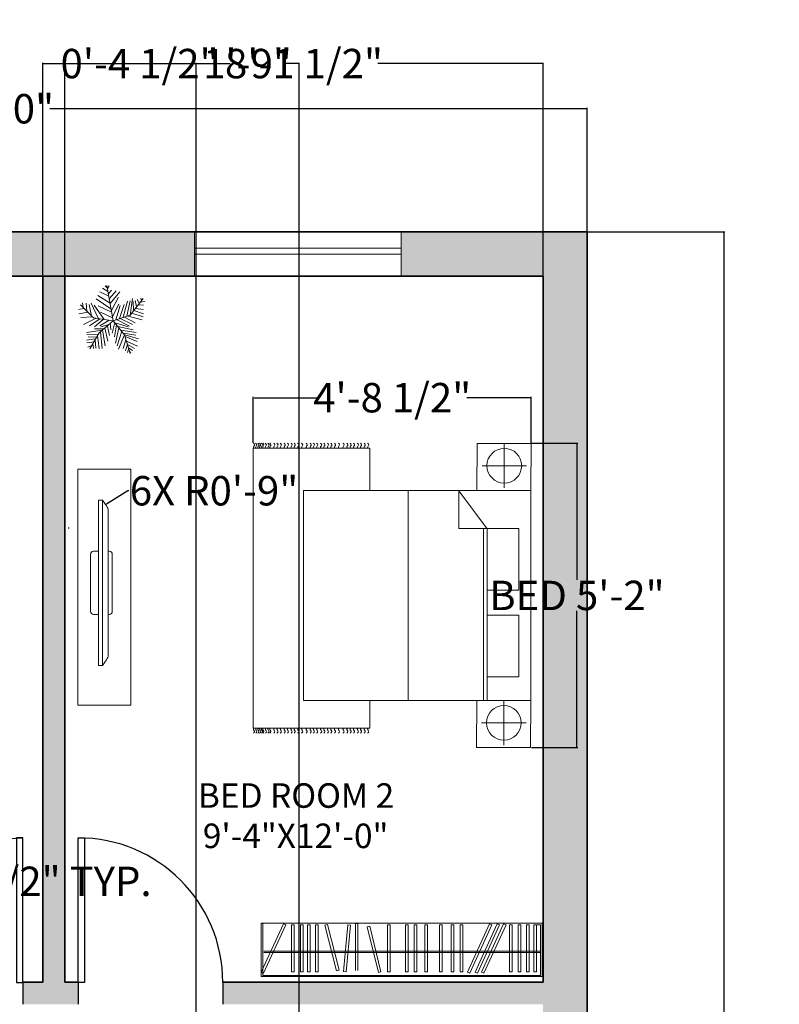
# Model space of a CAD drawing. Units: inches. Extents: x 143233372 to 143233714, y 112671713 to 112672292.
# Tile 7 of 7: x 143233541 to 143233695, y 112672092 to 112672292. Entities that reach past the tile are written whole.
import ezdxf

# ---------------------------------------------------------------- set-up
doc = ezdxf.new("R2010")
doc.units = ezdxf.units.IN
doc.header["$MEASUREMENT"] = 0
doc.layers.get('0').update_dxf_attribs({"color": 104})
for name, color, linetype, lineweight in [('A-ANNO-DIMS', 2, 'Continuous', 18), ('A-AREA-IDEN', 7, 'Continuous', 18), ('A-EQPM', 8, 'Continuous', 18), ('closet', 23, 'Continuous', 18), ('doors', 32, 'Continuous', 25), ('furniture', 23, 'Continuous', 18), ('L-PLNT', 92, 'Continuous', 13), ('walls', 7, 'Continuous', 35), ('windows', 4, 'Continuous', 18)]:
    doc.layers.add(name, color=color, linetype=linetype, lineweight=lineweight)
doc.layers.add('A-WALL-PATT', color=18, linetype='Continuous', lineweight=9, true_color=0x000000)
doc.styles.get("Standard").update_dxf_attribs({"font": 'arial.ttf'})
doc.dimstyles.get("Standard").update_dxf_attribs({"dimtxt": 6, "dimasz": 0.18, "dimexe": 0.18, "dimexo": 0.0625, "dimgap": 0.09, "dimtad": 0, "dimtih": 1, "dimtoh": 1, "dimzin": 0, "dimdsep": 46, "dimlunit": 3, "dimtxsty": 'Standard', "dimcen": 0.09, "dimadec": 0, "dimazin": 0, "dimtfac": 1, "dimtofl": 0, "dimtmove": 0, "dimatfit": 3, "dimfxl": 1, "dimtolj": 1, "dimtzin": 0, "dimarcsym": 0})

# ---------------------------------------------------------------- blocks, each defined once
blk = doc.blocks.new('PLASMA-LARGE')
at = {"layer": 'furniture'}
for p, q in [((-7.26, 0), (7.26, 0)), ((-21, -2.5), (21, -2.5)), ((-21, -2.5), (-21, -3.5)), ((-18.61, -1), (18.61, -1)), ((-8, -1), (-8, -0.74)), ((8, -1), (8, -0.74)), ((21, -2.5), (21, -3.5)), ((-21, -3.5), (21, -3.5)), ((-8, -3.5), (-8, -4.76)), ((8, -3.5), (8, -4.76)), ((-7.26, -5.5), (7.26, -5.5))]:
    blk.add_line(p, q, dxfattribs=at)
for centre, radius, start, end in [((-7.26, -0.74), 0.744, 90, 180), ((7.26, -0.74), 0.744, 0, 90), ((-13.97, -11.05), 11.07, 114.7602, 129.4175), ((13.97, -11.05), 11.07, 50.5825, 65.2398), ((-7.26, -4.76), 0.744, 180, 270), ((7.26, -4.76), 0.744, 270, 0)]:
    blk.add_arc(centre, radius, start, end, dxfattribs=at)
blk = doc.blocks.new('CARPET')
at = {"layer": 'furniture'}
for p, q in [((-51.53, -98.11), (-51.53, -55.12)), ((-51.53, -55.12), (-41.27, -55.12)), ((36, -55.12), (51.55, -55.12)), ((51.55, -55.12), (51.55, -98.11)), ((51.55, -98.11), (-51.53, -98.11))]:
    blk.add_line(p, q, dxfattribs=at)
for points, knots in [([(-53.37, -55.99), (-53.22, -55.8), (-52.9, -55.41), (-52.34, -55.8), (-51.89, -56.08), (-51.65, -55.91), (-51.53, -55.83)], [0, 0, 0, 0, 0.653278, 1.290138, 1.740457, 2.114451, 2.114451, 2.114451, 2.114451]), ([(-53.37, -57.26), (-53.22, -57.07), (-52.9, -56.67), (-52.34, -57.07), (-51.89, -57.35), (-51.65, -57.17), (-51.53, -57.1)], [0, 0, 0, 0, 0.653278, 1.290138, 1.740457, 2.114451, 2.114451, 2.114451, 2.114451]), ([(53.37, -55.99), (53.22, -55.8), (52.9, -55.41), (52.34, -55.8), (51.89, -56.08), (51.65, -55.91), (51.53, -55.83)], [0, 0, 0, 0, 0.653278, 1.290138, 1.740457, 2.114451, 2.114451, 2.114451, 2.114451]), ([(53.37, -57.26), (53.22, -57.07), (52.9, -56.67), (52.34, -57.07), (51.89, -57.35), (51.65, -57.17), (51.53, -57.1)], [0, 0, 0, 0, 0.653278, 1.290138, 1.740457, 2.114451, 2.114451, 2.114451, 2.114451]), ([(-53.37, -58.59), (-53.22, -58.4), (-52.9, -58.01), (-52.34, -58.4), (-51.89, -58.68), (-51.65, -58.5), (-51.53, -58.43)], [0, 0, 0, 0, 0.653278, 1.290138, 1.740457, 2.114451, 2.114451, 2.114451, 2.114451]), ([(-53.37, -59.78), (-53.22, -59.58), (-52.9, -59.19), (-52.34, -59.58), (-51.89, -59.86), (-51.65, -59.69), (-51.53, -59.61)], [0, 0, 0, 0, 0.653278, 1.290138, 1.740457, 2.114451, 2.114451, 2.114451, 2.114451]), ([(-53.37, -61.22), (-53.22, -61.02), (-52.9, -60.63), (-52.34, -61.02), (-51.89, -61.3), (-51.65, -61.13), (-51.53, -61.05)], [0, 0, 0, 0, 0.653278, 1.290138, 1.740457, 2.114451, 2.114451, 2.114451, 2.114451]), ([(53.37, -58.59), (53.22, -58.4), (52.9, -58.01), (52.34, -58.4), (51.89, -58.68), (51.65, -58.5), (51.53, -58.43)], [0, 0, 0, 0, 0.653278, 1.290138, 1.740457, 2.114451, 2.114451, 2.114451, 2.114451]), ([(53.37, -59.78), (53.22, -59.58), (52.9, -59.19), (52.34, -59.58), (51.89, -59.86), (51.65, -59.69), (51.53, -59.61)], [0, 0, 0, 0, 0.653278, 1.290138, 1.740457, 2.114451, 2.114451, 2.114451, 2.114451]), ([(53.37, -61.22), (53.22, -61.02), (52.9, -60.63), (52.34, -61.02), (51.89, -61.3), (51.65, -61.13), (51.53, -61.05)], [0, 0, 0, 0, 0.653278, 1.290138, 1.740457, 2.114451, 2.114451, 2.114451, 2.114451]), ([(-53.37, -62.44), (-53.22, -62.25), (-52.9, -61.86), (-52.34, -62.25), (-51.89, -62.53), (-51.65, -62.36), (-51.53, -62.28)], [0, 0, 0, 0, 0.653278, 1.290138, 1.740457, 2.114451, 2.114451, 2.114451, 2.114451]), ([(-53.37, -63.63), (-53.22, -63.43), (-52.9, -63.04), (-52.34, -63.43), (-51.89, -63.72), (-51.65, -63.54), (-51.53, -63.46)], [0, 0, 0, 0, 0.653278, 1.290138, 1.740457, 2.114451, 2.114451, 2.114451, 2.114451]), ([(-53.37, -65.07), (-53.22, -64.87), (-52.9, -64.48), (-52.34, -64.87), (-51.89, -65.15), (-51.65, -64.98), (-51.53, -64.9)], [0, 0, 0, 0, 0.653278, 1.290138, 1.740457, 2.114451, 2.114451, 2.114451, 2.114451]), ([(53.37, -62.44), (53.22, -62.25), (52.9, -61.86), (52.34, -62.25), (51.89, -62.53), (51.65, -62.36), (51.53, -62.28)], [0, 0, 0, 0, 0.653278, 1.290138, 1.740457, 2.114451, 2.114451, 2.114451, 2.114451]), ([(53.37, -63.63), (53.22, -63.43), (52.9, -63.04), (52.34, -63.43), (51.89, -63.72), (51.65, -63.54), (51.53, -63.46)], [0, 0, 0, 0, 0.653278, 1.290138, 1.740457, 2.114451, 2.114451, 2.114451, 2.114451]), ([(53.37, -65.07), (53.22, -64.87), (52.9, -64.48), (52.34, -64.87), (51.89, -65.15), (51.65, -64.98), (51.53, -64.9)], [0, 0, 0, 0, 0.653278, 1.290138, 1.740457, 2.114451, 2.114451, 2.114451, 2.114451]), ([(-53.37, -66.76), (-53.22, -66.56), (-52.9, -66.17), (-52.34, -66.56), (-51.89, -66.84), (-51.65, -66.67), (-51.53, -66.59)], [0, 0, 0, 0, 0.653278, 1.290138, 1.740457, 2.114451, 2.114451, 2.114451, 2.114451]), ([(-53.37, -68.2), (-53.22, -68), (-52.9, -67.61), (-52.34, -68), (-51.89, -68.28), (-51.65, -68.11), (-51.53, -68.03)], [0, 0, 0, 0, 0.653278, 1.290138, 1.740457, 2.114451, 2.114451, 2.114451, 2.114451]), ([(53.37, -66.76), (53.22, -66.56), (52.9, -66.17), (52.34, -66.56), (51.89, -66.84), (51.65, -66.67), (51.53, -66.59)], [0, 0, 0, 0, 0.653278, 1.290138, 1.740457, 2.114451, 2.114451, 2.114451, 2.114451]), ([(53.37, -68.2), (53.22, -68), (52.9, -67.61), (52.34, -68), (51.89, -68.28), (51.65, -68.11), (51.53, -68.03)], [0, 0, 0, 0, 0.653278, 1.290138, 1.740457, 2.114451, 2.114451, 2.114451, 2.114451]), ([(-53.37, -69.53), (-53.22, -69.33), (-52.9, -68.94), (-52.34, -69.33), (-51.89, -69.61), (-51.65, -69.44), (-51.53, -69.36)], [0, 0, 0, 0, 0.653278, 1.290138, 1.740457, 2.114451, 2.114451, 2.114451, 2.114451]), ([(-53.37, -70.79), (-53.22, -70.6), (-52.9, -70.21), (-52.34, -70.6), (-51.89, -70.88), (-51.65, -70.7), (-51.53, -70.63)], [0, 0, 0, 0, 0.653278, 1.290138, 1.740457, 2.114451, 2.114451, 2.114451, 2.114451]), ([(-53.37, -72.12), (-53.22, -71.93), (-52.9, -71.54), (-52.34, -71.93), (-51.89, -72.21), (-51.65, -72.04), (-51.53, -71.96)], [0, 0, 0, 0, 0.653278, 1.290138, 1.740457, 2.114451, 2.114451, 2.114451, 2.114451]), ([(53.37, -69.53), (53.22, -69.33), (52.9, -68.94), (52.34, -69.33), (51.89, -69.61), (51.65, -69.44), (51.53, -69.36)], [0, 0, 0, 0, 0.653278, 1.290138, 1.740457, 2.114451, 2.114451, 2.114451, 2.114451]), ([(53.37, -70.79), (53.22, -70.6), (52.9, -70.21), (52.34, -70.6), (51.89, -70.88), (51.65, -70.7), (51.53, -70.63)], [0, 0, 0, 0, 0.653278, 1.290138, 1.740457, 2.114451, 2.114451, 2.114451, 2.114451]), ([(53.37, -72.12), (53.22, -71.93), (52.9, -71.54), (52.34, -71.93), (51.89, -72.21), (51.65, -72.04), (51.53, -71.96)], [0, 0, 0, 0, 0.653278, 1.290138, 1.740457, 2.114451, 2.114451, 2.114451, 2.114451]), ([(-53.37, -73.31), (-53.22, -73.11), (-52.9, -72.72), (-52.34, -73.11), (-51.89, -73.4), (-51.65, -73.22), (-51.53, -73.14)], [0, 0, 0, 0, 0.653278, 1.290138, 1.740457, 2.114451, 2.114451, 2.114451, 2.114451]), ([(-53.37, -74.75), (-53.22, -74.55), (-52.9, -74.16), (-52.34, -74.55), (-51.89, -74.83), (-51.65, -74.66), (-51.53, -74.58)], [0, 0, 0, 0, 0.653278, 1.290138, 1.740457, 2.114451, 2.114451, 2.114451, 2.114451]), ([(-53.37, -75.98), (-53.22, -75.78), (-52.9, -75.39), (-52.34, -75.78), (-51.89, -76.06), (-51.65, -75.89), (-51.53, -75.81)], [0, 0, 0, 0, 0.653278, 1.290138, 1.740457, 2.114451, 2.114451, 2.114451, 2.114451]), ([(53.37, -73.31), (53.22, -73.11), (52.9, -72.72), (52.34, -73.11), (51.89, -73.4), (51.65, -73.22), (51.53, -73.14)], [0, 0, 0, 0, 0.653278, 1.290138, 1.740457, 2.114451, 2.114451, 2.114451, 2.114451]), ([(53.37, -74.75), (53.22, -74.55), (52.9, -74.16), (52.34, -74.55), (51.89, -74.83), (51.65, -74.66), (51.53, -74.58)], [0, 0, 0, 0, 0.653278, 1.290138, 1.740457, 2.114451, 2.114451, 2.114451, 2.114451]), ([(53.37, -75.98), (53.22, -75.78), (52.9, -75.39), (52.34, -75.78), (51.89, -76.06), (51.65, -75.89), (51.53, -75.81)], [0, 0, 0, 0, 0.653278, 1.290138, 1.740457, 2.114451, 2.114451, 2.114451, 2.114451]), ([(-53.37, -77.16), (-53.22, -76.96), (-52.9, -76.57), (-52.34, -76.96), (-51.89, -77.25), (-51.65, -77.07), (-51.53, -76.99)], [0, 0, 0, 0, 0.653278, 1.290138, 1.740457, 2.114451, 2.114451, 2.114451, 2.114451]), ([(-53.37, -78.6), (-53.22, -78.4), (-52.9, -78.01), (-52.34, -78.4), (-51.89, -78.68), (-51.65, -78.51), (-51.53, -78.43)], [0, 0, 0, 0, 0.653278, 1.290138, 1.740457, 2.114451, 2.114451, 2.114451, 2.114451]), ([(53.37, -77.16), (53.22, -76.96), (52.9, -76.57), (52.34, -76.96), (51.89, -77.25), (51.65, -77.07), (51.53, -76.99)], [0, 0, 0, 0, 0.653278, 1.290138, 1.740457, 2.114451, 2.114451, 2.114451, 2.114451]), ([(53.37, -78.6), (53.22, -78.4), (52.9, -78.01), (52.34, -78.4), (51.89, -78.68), (51.65, -78.51), (51.53, -78.43)], [0, 0, 0, 0, 0.653278, 1.290138, 1.740457, 2.114451, 2.114451, 2.114451, 2.114451]), ([(-53.37, -80.29), (-53.22, -80.09), (-52.9, -79.7), (-52.34, -80.09), (-51.89, -80.37), (-51.65, -80.2), (-51.53, -80.12)], [0, 0, 0, 0, 0.653278, 1.290138, 1.740457, 2.114451, 2.114451, 2.114451, 2.114451]), ([(-53.37, -81.73), (-53.22, -81.53), (-52.9, -81.14), (-52.34, -81.53), (-51.89, -81.81), (-51.65, -81.64), (-51.53, -81.56)], [0, 0, 0, 0, 0.653278, 1.290138, 1.740457, 2.114451, 2.114451, 2.114451, 2.114451]), ([(-53.37, -83.06), (-53.22, -82.86), (-52.9, -82.47), (-52.34, -82.86), (-51.89, -83.14), (-51.65, -82.97), (-51.53, -82.89)], [0, 0, 0, 0, 0.653278, 1.290138, 1.740457, 2.114451, 2.114451, 2.114451, 2.114451]), ([(53.37, -80.29), (53.22, -80.09), (52.9, -79.7), (52.34, -80.09), (51.89, -80.37), (51.65, -80.2), (51.53, -80.12)], [0, 0, 0, 0, 0.653278, 1.290138, 1.740457, 2.114451, 2.114451, 2.114451, 2.114451]), ([(53.37, -81.73), (53.22, -81.53), (52.9, -81.14), (52.34, -81.53), (51.89, -81.81), (51.65, -81.64), (51.53, -81.56)], [0, 0, 0, 0, 0.653278, 1.290138, 1.740457, 2.114451, 2.114451, 2.114451, 2.114451]), ([(53.37, -83.06), (53.22, -82.86), (52.9, -82.47), (52.34, -82.86), (51.89, -83.14), (51.65, -82.97), (51.53, -82.89)], [0, 0, 0, 0, 0.653278, 1.290138, 1.740457, 2.114451, 2.114451, 2.114451, 2.114451]), ([(-53.37, -84.18), (-53.22, -83.99), (-52.9, -83.6), (-52.34, -83.99), (-51.89, -84.27), (-51.65, -84.09), (-51.53, -84.02)], [0, 0, 0, 0, 0.653278, 1.290138, 1.740457, 2.114451, 2.114451, 2.114451, 2.114451]), ([(-53.37, -85.51), (-53.22, -85.32), (-52.9, -84.93), (-52.34, -85.32), (-51.89, -85.6), (-51.65, -85.42), (-51.53, -85.35)], [0, 0, 0, 0, 0.653278, 1.290138, 1.740457, 2.114451, 2.114451, 2.114451, 2.114451]), ([(-53.37, -86.7), (-53.22, -86.5), (-52.9, -86.11), (-52.34, -86.5), (-51.89, -86.78), (-51.65, -86.61), (-51.53, -86.53)], [0, 0, 0, 0, 0.653278, 1.290138, 1.740457, 2.114451, 2.114451, 2.114451, 2.114451]), ([(53.37, -84.18), (53.22, -83.99), (52.9, -83.6), (52.34, -83.99), (51.89, -84.27), (51.65, -84.09), (51.53, -84.02)], [0, 0, 0, 0, 0.653278, 1.290138, 1.740457, 2.114451, 2.114451, 2.114451, 2.114451]), ([(53.37, -85.51), (53.22, -85.32), (52.9, -84.93), (52.34, -85.32), (51.89, -85.6), (51.65, -85.42), (51.53, -85.35)], [0, 0, 0, 0, 0.653278, 1.290138, 1.740457, 2.114451, 2.114451, 2.114451, 2.114451]), ([(53.37, -86.7), (53.22, -86.5), (52.9, -86.11), (52.34, -86.5), (51.89, -86.78), (51.65, -86.61), (51.53, -86.53)], [0, 0, 0, 0, 0.653278, 1.290138, 1.740457, 2.114451, 2.114451, 2.114451, 2.114451]), ([(-53.37, -88.14), (-53.22, -87.94), (-52.9, -87.55), (-52.34, -87.94), (-51.89, -88.22), (-51.65, -88.05), (-51.53, -87.97)], [0, 0, 0, 0, 0.653278, 1.290138, 1.740457, 2.114451, 2.114451, 2.114451, 2.114451]), ([(-53.37, -89.36), (-53.22, -89.17), (-52.9, -88.78), (-52.34, -89.17), (-51.89, -89.45), (-51.65, -89.28), (-51.53, -89.2)], [0, 0, 0, 0, 0.653278, 1.290138, 1.740457, 2.114451, 2.114451, 2.114451, 2.114451]), ([(-53.37, -90.55), (-53.22, -90.35), (-52.9, -89.96), (-52.34, -90.35), (-51.89, -90.64), (-51.65, -90.46), (-51.53, -90.38)], [0, 0, 0, 0, 0.653278, 1.290138, 1.740457, 2.114451, 2.114451, 2.114451, 2.114451]), ([(53.37, -88.14), (53.22, -87.94), (52.9, -87.55), (52.34, -87.94), (51.89, -88.22), (51.65, -88.05), (51.53, -87.97)], [0, 0, 0, 0, 0.653278, 1.290138, 1.740457, 2.114451, 2.114451, 2.114451, 2.114451]), ([(53.37, -89.36), (53.22, -89.17), (52.9, -88.78), (52.34, -89.17), (51.89, -89.45), (51.65, -89.28), (51.53, -89.2)], [0, 0, 0, 0, 0.653278, 1.290138, 1.740457, 2.114451, 2.114451, 2.114451, 2.114451]), ([(53.37, -90.55), (53.22, -90.35), (52.9, -89.96), (52.34, -90.35), (51.9, -90.63), (51.66, -90.47), (51.55, -90.4)], [0, 0, 0, 0, 0.653278, 1.290138, 1.740457, 2.0926, 2.0926, 2.0926, 2.0926]), ([(-53.37, -91.99), (-53.22, -91.79), (-52.9, -91.4), (-52.34, -91.79), (-51.89, -92.07), (-51.65, -91.9), (-51.53, -91.82)], [0, 0, 0, 0, 0.653278, 1.290138, 1.740457, 2.114451, 2.114451, 2.114451, 2.114451]), ([(-53.37, -92.69), (-53.22, -92.48), (-52.9, -92.08), (-52.35, -92.49), (-51.89, -92.77), (-51.65, -92.6), (-51.53, -92.52)], [0, 0, 0, 0, 0.663904, 1.307406, 1.757725, 2.131719, 2.131719, 2.131719, 2.131719]), ([(-53.37, -93.61), (-53.22, -93.42), (-52.9, -93.03), (-52.34, -93.42), (-51.89, -93.7), (-51.65, -93.52), (-51.53, -93.45)], [0, 0, 0, 0, 0.653278, 1.290138, 1.740457, 2.114451, 2.114451, 2.114451, 2.114451]), ([(-53.37, -94.55), (-53.22, -94.35), (-52.9, -93.96), (-52.34, -94.35), (-51.89, -94.63), (-51.65, -94.46), (-51.53, -94.38)], [0, 0, 0, 0, 0.653278, 1.290138, 1.740457, 2.114451, 2.114451, 2.114451, 2.114451]), ([(53.37, -91.99), (53.22, -91.79), (52.9, -91.4), (52.34, -91.79), (51.9, -92.07), (51.66, -91.91), (51.55, -91.83)], [0, 0, 0, 0, 0.653278, 1.290138, 1.740457, 2.0926, 2.0926, 2.0926, 2.0926]), ([(53.37, -92.69), (53.22, -92.49), (52.9, -92.09), (52.34, -92.49), (51.9, -92.77), (51.66, -92.61), (51.55, -92.53)], [0, 0, 0, 0, 0.656792, 1.295826, 1.746145, 2.098292, 2.098292, 2.098292, 2.098292]), ([(53.37, -93.66), (53.22, -93.46), (52.9, -93.07), (52.34, -93.46), (51.9, -93.74), (51.66, -93.58), (51.55, -93.5)], [0, 0, 0, 0, 0.653278, 1.290138, 1.740457, 2.0926, 2.0926, 2.0926, 2.0926]), ([(53.37, -94.59), (53.22, -94.4), (52.9, -94.01), (52.34, -94.4), (51.9, -94.68), (51.66, -94.51), (51.55, -94.44)], [0, 0, 0, 0, 0.653278, 1.290138, 1.740457, 2.0926, 2.0926, 2.0926, 2.0926]), ([(-53.37, -95.05), (-53.22, -94.85), (-52.9, -94.46), (-52.34, -94.85), (-51.89, -95.14), (-51.65, -94.96), (-51.53, -94.88)], [0, 0, 0, 0, 0.653278, 1.290138, 1.740457, 2.114451, 2.114451, 2.114451, 2.114451]), ([(-53.37, -95.73), (-53.22, -95.54), (-52.9, -95.15), (-52.34, -95.54), (-51.89, -95.82), (-51.65, -95.65), (-51.53, -95.57)], [0, 0, 0, 0, 0.653278, 1.290138, 1.740457, 2.114451, 2.114451, 2.114451, 2.114451]), ([(-53.37, -96.38), (-53.22, -96.18), (-52.9, -95.79), (-52.34, -96.18), (-51.89, -96.47), (-51.65, -96.29), (-51.53, -96.21)], [0, 0, 0, 0, 0.653278, 1.290138, 1.740457, 2.114451, 2.114451, 2.114451, 2.114451]), ([(-53.37, -97.17), (-53.22, -96.98), (-52.9, -96.59), (-52.34, -96.98), (-51.89, -97.26), (-51.65, -97.08), (-51.53, -97.01)], [0, 0, 0, 0, 0.653278, 1.290138, 1.740457, 2.114451, 2.114451, 2.114451, 2.114451]), ([(-53.37, -97.99), (-53.22, -97.79), (-52.9, -97.4), (-52.34, -97.79), (-51.89, -98.08), (-51.65, -97.9), (-51.53, -97.82)], [0, 0, 0, 0, 0.653278, 1.290138, 1.740457, 2.114451, 2.114451, 2.114451, 2.114451]), ([(53.37, -95.78), (53.22, -95.58), (52.9, -95.19), (52.34, -95.58), (51.89, -95.86), (51.65, -95.69), (51.53, -95.61)], [0, 0, 0, 0, 0.653278, 1.290138, 1.740457, 2.114451, 2.114451, 2.114451, 2.114451]), ([(53.37, -96.43), (53.22, -96.23), (52.9, -95.84), (52.34, -96.23), (51.89, -96.51), (51.65, -96.34), (51.53, -96.26)], [0, 0, 0, 0, 0.653278, 1.290138, 1.740457, 2.114451, 2.114451, 2.114451, 2.114451]), ([(53.37, -97.22), (53.22, -97.02), (52.9, -96.63), (52.34, -97.02), (51.89, -97.3), (51.65, -97.13), (51.53, -97.05)], [0, 0, 0, 0, 0.653278, 1.290138, 1.740457, 2.114451, 2.114451, 2.114451, 2.114451]), ([(53.37, -97.99), (53.22, -97.79), (52.9, -97.4), (52.34, -97.79), (51.89, -98.08), (51.65, -97.9), (51.53, -97.82)], [0, 0, 0, 0, 0.653278, 1.290138, 1.740457, 2.114451, 2.114451, 2.114451, 2.114451]), ([(53.37, -95.1), (53.22, -94.9), (52.9, -94.51), (52.34, -94.9), (51.9, -95.18), (51.66, -95.02), (51.55, -94.94)], [0, 0, 0, 0, 0.653278, 1.290138, 1.740457, 2.0926, 2.0926, 2.0926, 2.0926])]:
    blk.add_open_spline(points, degree=3, knots=knots, dxfattribs=at)
blk = doc.blocks.new('A$C58D270C6')
at = {"layer": 'furniture'}
for p, q in [((9.09, 124.13), (9.09, 108.87)), ((1.46, 116.5), (16.73, 116.5)), ((14.97, 94.84), (24.62, 107.92)), ((24.62, 94.93), (24.62, 107.92)), ((42.08, 108), (42.08, 36)), ((14.97, 94.93), (24.62, 94.93)), ((14.97, 94.84), (14.97, 36)), ((16.22, 94.93), (16.22, 36)), ((9.25, 36), (9.25, 20.74)), ((1.62, 28.37), (16.88, 28.37))]:
    blk.add_line(p, q, dxfattribs=at)
for points in [[(18.5, 108), (18.34, 124.13), (-0.16, 124.13), (0, 108)], [(0, 108), (77.91, 108), (77.91, 36), (0, 36)], [(4.09, 94.93), (14.97, 94.93), (14.97, 73.83), (4.09, 73.83)], [(4.09, 65.23), (14.97, 65.23), (14.97, 44.13), (4.09, 44.13)], [(18.65, 19.87), (18.5, 36), (0, 36), (0.16, 19.87)]]:
    blk.add_lwpolyline(points, close=True, dxfattribs=at)
for centre in [(9.09, 116.5), (9.25, 28.37)]:
    blk.add_circle(centre, 5.95, dxfattribs=at)
at = {"layer": 'furniture', "xscale": 0.9312884925094044, "yscale": 0.9312884925094044, "zscale": 0.9312884925094044, "rotation": 90}
blk.add_blockref('CARPET', (3.79, 74.47), dxfattribs=at)
blk = doc.blocks.new('closet')
at = {"layer": 'closet'}
for p, q in [((-0.71, -5.58), (5.59, 8.19)), ((-0.23, 7.39), (-0.23, -6.57)), ((6.27, 7.88), (-0.04, -5.89)), ((5.59, 8.19), (6.27, 7.88)), ((7.92, 7.84), (8.68, 7.84)), ((7.92, 7.84), (7.92, -5.51)), ((8.68, 7.84), (8.68, -5.51)), ((10.44, 7.84), (11.2, 7.84)), ((10.44, 7.84), (10.44, -5.51)), ((11.2, 7.84), (11.2, -5.51)), ((12.45, 7.84), (13.21, 7.84)), ((12.45, 7.84), (12.45, -5.51)), ((13.21, 7.84), (13.21, -5.51)), ((14.71, 7.84), (15.47, 7.84)), ((14.71, 7.84), (14.71, -5.51)), ((15.47, 7.84), (15.47, -5.51)), ((17.44, 7.75), (18.17, 7.93)), ((17.44, 7.75), (20.73, -5.2)), ((18.17, 7.93), (21.46, -5.01)), ((23.92, 7.84), (22.75, -5.46)), ((24.67, 7.78), (23.51, -5.53)), ((23.92, 7.84), (24.67, 7.78)), ((26.09, 8.25), (26.09, -5.1)), ((26.84, 8.25), (26.84, -5.1)), ((29.49, 7.29), (32.64, -5.69)), ((30.22, 7.46), (33.37, -5.51)), ((35.23, 7.84), (35.23, -5.51)), ((35.99, 7.84), (35.99, -5.51)), ((40.33, 7.84), (40.33, -5.51)), ((41.08, 7.84), (41.08, -5.51)), ((42.85, 7.84), (42.85, -5.51)), ((43.61, 7.84), (43.61, -5.51)), ((45.9, 7.84), (45.9, -5.51)), ((46.65, 7.84), (46.65, -5.51)), ((50.07, 7.84), (50.07, -5.51)), ((50.82, 7.84), (50.82, -5.51)), ((53.32, 7.84), (53.32, -5.51)), ((54.08, 7.84), (54.08, -5.51)), ((55.9, 7.84), (55.9, -5.51)), ((56.65, 7.84), (56.65, -5.51)), ((57.99, -5.58), (64.3, 8.19)), ((64.97, 7.88), (58.67, -5.89)), ((60.19, -5.58), (66.49, 8.19)), ((67.17, 7.88), (60.87, -5.89)), ((62, -5.58), (68.3, 8.19)), ((68.98, 7.88), (62.67, -5.89)), ((69.96, 7.84), (69.96, -5.51)), ((70.72, 7.84), (70.72, -5.51)), ((72.43, 7.84), (72.43, -5.51)), ((73.19, 7.84), (73.19, -5.51)), ((74.82, 7.84), (74.82, -5.51)), ((75.57, 7.84), (75.57, -5.51)), ((76.94, 7.84), (76.94, -5.51)), ((77.69, 7.84), (77.69, -5.51)), ((56.23, 0.33), (0, 0.33)), ((56.2, 0), (0, 0)), ((56.2, 0), (78.76, 0)), ((56.23, 0.33), (78.76, 0.33)), ((-0.04, -5.89), (-0.71, -5.58)), ((21.46, -5.01), (20.73, -5.2)), ((23.51, -5.53), (22.75, -5.46)), ((33.37, -5.51), (32.64, -5.69)), ((35.99, -5.51), (35.23, -5.51)), ((41.08, -5.51), (40.33, -5.51)), ((43.61, -5.51), (42.85, -5.51)), ((46.65, -5.51), (45.9, -5.51)), ((50.82, -5.51), (50.07, -5.51)), ((54.08, -5.51), (53.32, -5.51)), ((56.65, -5.51), (55.9, -5.51)), ((58.67, -5.89), (57.99, -5.58)), ((60.87, -5.89), (60.19, -5.58)), ((62.67, -5.89), (62, -5.58)), ((70.72, -5.51), (69.96, -5.51)), ((73.19, -5.51), (72.43, -5.51)), ((75.57, -5.51), (74.82, -5.51)), ((77.69, -5.51), (76.94, -5.51))]:
    blk.add_line(p, q, dxfattribs=at)
blk = doc.blocks.new('rotated closet')
at = {"layer": 'closet'}
for p, q in [((26.32, 0.86), (27.07, 0.86)), ((29.72, -0.11), (30.45, 0.07)), ((35.46, 0.45), (36.22, 0.45)), ((40.56, 0.45), (41.31, 0.45)), ((43.08, 0.45), (43.84, 0.45)), ((46.13, 0.45), (46.88, 0.45)), ((50.3, 0.45), (51.05, 0.45)), ((53.56, 0.45), (54.31, 0.45)), ((56.13, 0.45), (56.88, 0.45)), ((64.53, 0.8), (65.2, 0.49)), ((66.72, 0.8), (67.4, 0.49)), ((68.53, 0.8), (69.21, 0.49)), ((70.19, 0.45), (70.95, 0.45)), ((72.66, 0.45), (73.42, 0.45)), ((75.05, 0.45), (75.81, 0.45)), ((77.17, 0.45), (77.92, 0.45)), ((78.99, 0), (78.99, -13.96)), ((0, -13.96), (78.99, -13.96)), ((8.91, -12.91), (8.15, -12.91)), ((11.43, -12.91), (10.67, -12.91)), ((13.44, -12.91), (12.68, -12.91)), ((15.7, -12.91), (14.94, -12.91)), ((-0.46, -14.27), (79.54, -14.27))]:
    blk.add_line(p, q, dxfattribs=at)
blk.add_blockref('closet', (0.23, -7.39), dxfattribs=at)
blk = doc.blocks.new('*U24')
for p, q in [((0, 0), (0, -6)), ((40, 0), (40, -6))]:
    blk.add_line(p, q)
blk.add_lwpolyline([(0, 0), (0, 40), (1.75, 40), (1.75, 0)], close=True)
blk.add_arc((0, 0), 40, 0, 90)
blk = doc.blocks.new('*U26')
for p, q in [((-8.737, 47.138), (-17.069, 52.711)), ((-10.186, 53.64), (-13.084, 55.962)), ((0, 0), (-10.5, 57)), ((-9.099, 51.782), (-6.563, 55.962)), ((-7.65, 43.423), (-2.578, 49.46)), ((-5.839, 35.992), (4.667, 48.067)), ((-3.665, 19.273), (-27.574, 35.527)), ((-5.114, 28.097), (-24.676, 40.636)), ((-7.288, 39.707), (-21.778, 46.673)), ((-5.114, 27.632), (10.463, 46.673)), ((-2.941, 16.486), (8.652, 37.85)), ((22.055, 7.198), (27.489, 32.277)), ((27, 9), (48, 36)), ((27.127, 9.056), (31.112, 35.992)), ((35.096, 32.741), (37.27, 22.524)), ((38.719, 34.134), (41.979, 28.561)), ((44.153, 36.456), (45.239, 32.741)), ((-47.498, 19.737), (-55.83, 18.344)), ((-31.5, 4.5), (-52.5, 25.5)), ((-48.585, 21.131), (-49.309, 29.026)), ((-43.513, 28.561), (-42.427, 15.558)), ((-38.442, 26.239), (-34.819, 7.663)), ((-35.544, 28.097), (-24.314, 3.947)), ((-14.533, 2.09), (-30.834, 25.31)), ((-24.314, 23.917), (-2.941, 13.7)), ((-1.129, 6.734), (9.014, 26.704)), ((3.942, 1.625), (11.187, 24.381)), ((10.101, 3.483), (17.708, 26.239)), ((16.259, 5.805), (23.142, 31.348)), ((31.836, 30.883), (32.561, 16.486)), ((33.285, 16.486), (48.862, 10.913)), ((36.183, 19.737), (48.137, 17.88)), ((40.53, 25.775), (48.862, 24.846)), ((43.791, 29.954), (51.036, 30.883)), ((-40.615, 13.7), (-55.105, 10.913)), ((-33.37, 6.269), (-52.207, 5.34)), ((-28.299, 3.483), (-47.86, -5.805)), ((-21.416, 3.018), (-38.079, -8.128)), ((0, 0), (-31.5, 4.5)), ((-15.982, 2.09), (-30.11, -9.521)), ((0, 0), (-22.5, -19.5)), ((-6.563, 1.161), (-21.416, -8.128)), ((-20.691, 13.7), (-1.129, 4.876)), ((0, 0), (27, 9)), ((0, 0), (18, -22.5)), ((6.478, 1.625), (26.04, -8.592)), ((11.187, 3.483), (30.749, -5.805)), ((18.07, 5.805), (35.096, -3.483)), ((24.229, 7.663), (46.688, 1.625)), ((29.662, 12.307), (48.137, 6.269)), ((-17.431, -15.094), (-42.789, -18.809)), ((-15.257, -12.772), (-30.11, -12.772)), ((-6.563, -5.805), (-19.967, -9.985)), ((-17.069, -15.094), (-12.721, -40.172)), ((-13.446, -11.378), (-8.737, -32.741)), ((-9.461, -8.592), (-6.201, -23.453)), ((-4.752, -3.483), (-3.665, -14.629)), ((2.493, -3.019), (-1.491, -20.202)), ((1.769, -2.555), (24.229, -9.521)), ((5.029, -6.27), (2.131, -25.775)), ((9.014, -11.378), (3.58, -35.992)), ((7.565, -9.056), (32.198, -14.629)), ((12.274, -15.094), (36.907, -18.809)), ((-28.299, -29.026), (-42.789, -31.348)), ((-24.314, -21.596), (-42.427, -22.06)), ((-26.849, -26.24), (-40.253, -25.775)), ((-22.5, -19.5), (-37.5, -45)), ((-29.023, -30.884), (-27.936, -43.887)), ((-25.038, -23.918), (-22.865, -45.281)), ((-20.691, -18.345), (-17.793, -44.352)), ((14.085, -16.951), (6.478, -40.172)), ((18.07, -22.524), (8.289, -45.745)), ((20.244, -30.419), (15.897, -44.816)), ((16.259, -19.738), (36.183, -22.989)), ((18, -22.5), (27, -52.5)), ((18.433, -22.524), (40.53, -29.026)), ((19.157, -25.311), (38.719, -33.206)), ((-30.834, -34.135), (-42.427, -35.528)), ((-34.457, -39.708), (-40.978, -42.494)), ((-32.646, -36.921), (-31.921, -44.352)), ((22.78, -37.85), (19.519, -48.532)), ((21.331, -32.741), (39.081, -40.636)), ((22.78, -38.314), (34.372, -44.816)), ((24.591, -45.745), (23.142, -50.854)), ((24.591, -43.423), (30.749, -47.603)), ((26.764, -49.925), (28.213, -50.854))]:
    blk.add_line(p, q)
blk = doc.blocks.new('*D27')
at = {"layer": 'A-ANNO-DIMS', "color": 0, "lineweight": -2, "transparency": 16777216}
for p, q in [((143233416.28, 112672249.24), (143233416.28, 112672274.49)), ((143233416.46, 112672274.31), (143233525.84, 112672274.31)), ((143233656.1, 112672274.31), (143233546.73, 112672274.31)), ((143233656.28, 112672249.24), (143233656.28, 112672274.49))]:
    blk.add_line(p, q, dxfattribs=at)
at = {"layer": 'A-ANNO-DIMS', "color": 0, "transparency": 16777216}
for points in [[(143233416.46, 112672274.34), (143233416.46, 112672274.28), (143233416.28, 112672274.31)], [(143233656.1, 112672274.34), (143233656.1, 112672274.28), (143233656.28, 112672274.31)]]:
    blk.add_solid(points, dxfattribs=at)
at = {"layer": 'Defpoints', "color": 0, "transparency": 16777216}
for p in [(143233656.28, 112672274.31), (143233416.28, 112672249.18), (143233656.28, 112672249.18)]:
    blk.add_point(p, dxfattribs=at)
at = {"layer": 'A-ANNO-DIMS', "color": 0, "transparency": 16777216, "insert": (143233536.28, 112672274.31), "char_height": 6, "attachment_point": 5}
blk.add_mtext('\\A1;20\'-0"', dxfattribs=at)
blk = doc.blocks.new('SASH-42IN')
for p, q in [((0, 1.17), (42.12, 1.17)), ((42.12, 0), (0, 0)), ((42.12, 1.17), (42.12, 0))]:
    blk.add_line(p, q)
blk = doc.blocks.new('MEDIA-CONSOLE')
for p, q in [((0, 48.12), (10.82, 48.12)), ((0, 0), (0, 48.12)), ((10.82, 48.12), (10.82, 0)), ((10.82, 0), (0, 0))]:
    blk.add_line(p, q)
blk = doc.blocks.new('*D43')
at = {"layer": 'A-ANNO-DIMS', "color": 0, "lineweight": -2, "transparency": 16777216}
for p, q in [((143233644.93, 112672206.09), (143233654.36, 112672206.09)), ((143233654.18, 112672205.91), (143233654.18, 112672178.22)), ((143233654.18, 112672144.22), (143233654.18, 112672171.91)), ((143233644.93, 112672144.04), (143233654.36, 112672144.04))]:
    blk.add_line(p, q, dxfattribs=at)
at = {"layer": 'A-ANNO-DIMS', "color": 0, "transparency": 16777216}
for points in [[(143233654.15, 112672205.91), (143233654.21, 112672205.91), (143233654.18, 112672206.09)], [(143233654.15, 112672144.22), (143233654.21, 112672144.22), (143233654.18, 112672144.04)]]:
    blk.add_solid(points, dxfattribs=at)
at = {"layer": 'Defpoints', "color": 0, "transparency": 16777216}
for p in [(143233644.87, 112672206.09), (143233654.18, 112672206.09), (143233644.87, 112672144.04)]:
    blk.add_point(p, dxfattribs=at)
at = {"layer": 'A-ANNO-DIMS', "color": 0, "transparency": 16777216, "insert": (143233654.18, 112672175.06), "char_height": 6, "attachment_point": 5}
blk.add_mtext('\\A1;BED 5\'-2"', dxfattribs=at)
blk = doc.blocks.new('*D44')
at = {"layer": 'A-ANNO-DIMS', "color": 0, "lineweight": -2, "transparency": 16777216}
for p, q in [((143233588.17, 112672206.15), (143233588.17, 112672215.57)), ((143233588.35, 112672215.39), (143233601.35, 112672215.39)), ((143233644.69, 112672215.39), (143233631.7, 112672215.39)), ((143233644.87, 112672206.15), (143233644.87, 112672215.57))]:
    blk.add_line(p, q, dxfattribs=at)
at = {"layer": 'A-ANNO-DIMS', "color": 0, "transparency": 16777216}
for points in [[(143233588.35, 112672215.42), (143233588.35, 112672215.36), (143233588.17, 112672215.39)], [(143233644.69, 112672215.42), (143233644.69, 112672215.36), (143233644.87, 112672215.39)]]:
    blk.add_solid(points, dxfattribs=at)
at = {"layer": 'Defpoints', "color": 0, "transparency": 16777216}
for p in [(143233588.17, 112672215.39), (143233588.17, 112672206.09), (143233644.87, 112672206.09)]:
    blk.add_point(p, dxfattribs=at)
at = {"layer": 'A-ANNO-DIMS', "color": 0, "transparency": 16777216, "insert": (143233616.52, 112672215.39), "char_height": 6, "attachment_point": 5}
blk.add_mtext('\\A1;4\'-8 1/2"', dxfattribs=at)
blk = doc.blocks.new('*D47')
at = {"layer": 'A-ANNO-DIMS', "color": 0, "lineweight": -2, "transparency": 16777216}
for p, q in [((143233425.27, 112672108.23), (143233425.27, 112672116.94)), ((143233425.45, 112672116.76), (143233482.38, 112672116.76)), ((143233482.56, 112672108.23), (143233482.56, 112672116.94)), ((143233482.56, 112672116.76), (143233482.74, 112672116.76))]:
    blk.add_line(p, q, dxfattribs=at)
at = {"layer": 'A-ANNO-DIMS', "color": 0, "transparency": 16777216}
for points in [[(143233425.45, 112672116.79), (143233425.45, 112672116.73), (143233425.27, 112672116.76)], [(143233482.38, 112672116.79), (143233482.38, 112672116.73), (143233482.56, 112672116.76)]]:
    blk.add_solid(points, dxfattribs=at)
at = {"layer": 'Defpoints', "color": 0, "transparency": 16777216}
for p in [(143233482.56, 112672116.76), (143233425.27, 112672108.17), (143233482.56, 112672108.17)]:
    blk.add_point(p, dxfattribs=at)
at = {"layer": 'A-ANNO-DIMS', "color": 0, "transparency": 16777216, "insert": (143233526.01, 112672116.76), "char_height": 6, "attachment_point": 5}
blk.add_mtext('\\A1;CLOSET 4\'-9 1/2" TYP.', dxfattribs=at)
blk = doc.blocks.new('*D63')
at = {"layer": 'A-ANNO-DIMS', "color": 0, "lineweight": -2, "transparency": 16777216}
for p, q in [((143233656.35, 112672249.18), (143233684.29, 112672249.18)), ((143233684.11, 112672249), (143233684.11, 112671999.82)), ((143233684.11, 112671744.43), (143233684.11, 112671993.61)), ((143233656.35, 112671744.25), (143233684.29, 112671744.25))]:
    blk.add_line(p, q, dxfattribs=at)
at = {"layer": 'A-ANNO-DIMS', "color": 0, "transparency": 16777216}
for points in [[(143233684.08, 112672249), (143233684.14, 112672249), (143233684.11, 112672249.18)], [(143233684.08, 112671744.43), (143233684.14, 112671744.43), (143233684.11, 112671744.25)]]:
    blk.add_solid(points, dxfattribs=at)
at = {"layer": 'Defpoints', "color": 0, "transparency": 16777216}
for p in [(143233656.28, 112672249.18), (143233656.28, 112671744.25), (143233684.11, 112671744.25)]:
    blk.add_point(p, dxfattribs=at)
at = {"layer": 'A-ANNO-DIMS', "color": 0, "transparency": 16777216, "insert": (143233684.11, 112671996.72), "char_height": 6, "attachment_point": 5}
blk.add_mtext('\\A1;42\'-1"', dxfattribs=at)
blk = doc.blocks.new('*D65')
at = {"layer": 'A-ANNO-DIMS', "color": 0, "lineweight": -2, "transparency": 16777216}
for p, q in [((143233545.28, 112672240.24), (143233545.28, 112672283.7)), ((143233545.46, 112672283.52), (143233549.6, 112672283.52)), ((143233549.78, 112672240.24), (143233549.78, 112672283.7)), ((143233549.78, 112672283.52), (143233549.96, 112672283.52))]:
    blk.add_line(p, q, dxfattribs=at)
at = {"layer": 'A-ANNO-DIMS', "color": 0, "transparency": 16777216}
for points in [[(143233545.46, 112672283.55), (143233545.46, 112672283.49), (143233545.28, 112672283.52)], [(143233549.6, 112672283.55), (143233549.6, 112672283.49), (143233549.78, 112672283.52)]]:
    blk.add_solid(points, dxfattribs=at)
at = {"layer": 'Defpoints', "color": 0, "transparency": 16777216}
for p in [(143233549.78, 112672283.52), (143233545.28, 112672240.18), (143233549.78, 112672240.18)]:
    blk.add_point(p, dxfattribs=at)
at = {"layer": 'A-ANNO-DIMS', "color": 0, "transparency": 16777216, "insert": (143233565.02, 112672283.52), "char_height": 6, "attachment_point": 5}
blk.add_mtext('\\A1;0\'-4 1/2"', dxfattribs=at)
blk = doc.blocks.new('*D66')
at = {"layer": 'A-ANNO-DIMS', "color": 0, "lineweight": -2, "transparency": 16777216}
for p, q in [((143233549.78, 112672240.24), (143233549.78, 112672283.7)), ((143233549.96, 112672283.52), (143233583.48, 112672283.52)), ((143233647.1, 112672283.52), (143233613.59, 112672283.52)), ((143233647.28, 112672240.24), (143233647.28, 112672283.7))]:
    blk.add_line(p, q, dxfattribs=at)
at = {"layer": 'A-ANNO-DIMS', "color": 0, "transparency": 16777216}
for points in [[(143233549.96, 112672283.55), (143233549.96, 112672283.49), (143233549.78, 112672283.52)], [(143233647.1, 112672283.55), (143233647.1, 112672283.49), (143233647.28, 112672283.52)]]:
    blk.add_solid(points, dxfattribs=at)
at = {"layer": 'Defpoints', "color": 0, "transparency": 16777216}
for p in [(143233647.28, 112672283.52), (143233549.78, 112672240.18), (143233647.28, 112672240.18)]:
    blk.add_point(p, dxfattribs=at)
at = {"layer": 'A-ANNO-DIMS', "color": 0, "transparency": 16777216, "insert": (143233598.53, 112672283.52), "char_height": 6, "attachment_point": 5}
blk.add_mtext('\\A1;8\'-1 1/2"', dxfattribs=at)
blk = doc.blocks.new('*D71')
at = {"layer": 'A-ANNO-DIMS', "color": 0, "lineweight": -2, "transparency": 16777216}
for p, q in [((143233576.53, 112672062.74), (143233576.53, 112672283.7)), ((143233576.71, 112672283.52), (143233579.24, 112672283.52)), ((143233597.35, 112672283.52), (143233594.81, 112672283.52)), ((143233597.53, 112672062.74), (143233597.53, 112672283.7))]:
    blk.add_line(p, q, dxfattribs=at)
at = {"layer": 'A-ANNO-DIMS', "color": 0, "transparency": 16777216}
for points in [[(143233576.71, 112672283.55), (143233576.71, 112672283.49), (143233576.53, 112672283.52)], [(143233597.35, 112672283.55), (143233597.35, 112672283.49), (143233597.53, 112672283.52)]]:
    blk.add_solid(points, dxfattribs=at)
at = {"layer": 'Defpoints', "color": 0, "transparency": 16777216}
for p in [(143233597.53, 112672283.52), (143233576.53, 112672062.68), (143233597.53, 112672062.68)]:
    blk.add_point(p, dxfattribs=at)
at = {"layer": 'A-ANNO-DIMS', "color": 0, "transparency": 16777216, "insert": (143233587.03, 112672283.52), "char_height": 6, "attachment_point": 5}
blk.add_mtext('\\A1;1\'-9"', dxfattribs=at)
blk = doc.blocks.new('*D77')
at = {"layer": 'A-ANNO-DIMS', "color": 0, "lineweight": -2, "transparency": 16777216}
for p, q in [((143233562.62, 112672196.41), (143233558.25, 112672193.67)), ((143233562.8, 112672196.41), (143233562.62, 112672196.41)), ((143233550.48, 112672188.85), (143233550.66, 112672188.85)), ((143233550.57, 112672188.76), (143233550.57, 112672188.94))]:
    blk.add_line(p, q, dxfattribs=at)
at = {"layer": 'A-ANNO-DIMS', "color": 0, "transparency": 16777216}
blk.add_solid([(143233558.24, 112672193.7), (143233558.27, 112672193.65), (143233558.1, 112672193.57)], dxfattribs=at)
at = {"layer": 'Defpoints', "color": 0, "transparency": 16777216}
for p in [(143233558.1, 112672193.57), (143233550.57, 112672188.85)]:
    blk.add_point(p, dxfattribs=at)
at = {"layer": 'A-ANNO-DIMS', "color": 0, "transparency": 16777216, "insert": (143233580.2, 112672196.41), "char_height": 6, "attachment_point": 5}
blk.add_mtext('\\A1;6X R0\'-9"', dxfattribs=at)

msp = doc.modelspace()

# ---------------------------------------------------------------- hatches: boundary and pattern name
at = {"layer": 'A-WALL-PATT'}
h = msp.add_hatch(color=256, dxfattribs=at)
h.dxf.hatch_style = 1
h.paths.add_polyline_path([(143233425.285, 112671820.328), (143233416.222, 112671820.328), (143233416.222, 112671767.682), (143233464.805, 112671767.682), (143233464.805, 112671776.682), (143233425.285, 112671776.682)])
h.paths.add_polyline_path([(143233425.285, 112672055.48), (143233416.285, 112672055.48), (143233416.285, 112671984.159), (143233425.285, 112671984.159)])
h.paths.add_polyline_path([(143233656.285, 112671963.912), (143233647.285, 112671963.912), (143233647.285, 112671848.682), (143233647.285, 112671839.682), (143233656.285, 112671839.682), (143233656.285, 112671889.182)])
h.paths.add_polyline_path([(143233425.285, 112672097.332), (143233425.285, 112672097.332), (143233425.285, 112672108.216), (143233425.285, 112672240.182), (143233451.497, 112672240.182), (143233451.497, 112672249.182), (143233416.285, 112672249.182), (143233416.285, 112672079.453), (143233420.069, 112672079.453), (143233425.285, 112672079.453)])
h.paths.add_polyline_path([(143233576.214, 112672249.182), (143233493.616, 112672249.182), (143233493.616, 112672240.182), (143233576.214, 112672240.182)])
h.paths.add_polyline_path([(143233425.285, 112671942.039), (143233416.285, 112671942.039), (143233416.285, 112671889.182), (143233416.271, 112671862.447), (143233425.285, 112671862.447), (143233425.285, 112671896.682), (143233518.63, 112671896.682, -0.0122006), (143233518.603, 112671897.787), (143233518.603, 112671901.182), (143233425.285, 112671901.182)])
h = msp.add_hatch(color=256, dxfattribs=at)
h.dxf.hatch_style = 1
h.paths.add_polyline_path([(143233656.285, 112672249.182), (143233647.285, 112672249.182), (143233647.285, 112672240.182), (143233656.285, 112672240.182)])
h.paths.add_polyline_path([(143233647.285, 112672249.182), (143233618.333, 112672249.182), (143233618.333, 112672240.182), (143233647.285, 112672240.182)])
h.paths.add_polyline_path([(143233656.285, 112672240.182), (143233647.285, 112672240.182), (143233647.285, 112672096.182), (143233656.285, 112672096.182)])
h.paths.add_polyline_path([(143233656.285, 112672096.182), (143233647.285, 112672096.182), (143233647.285, 112672091.682), (143233656.285, 112672091.682)])
h.paths.add_polyline_path([(143233647.285, 112672096.182), (143233581.998, 112672096.182), (143233581.998, 112672091.682), (143233647.285, 112672091.682)])
h.paths.add_polyline_path([(143233656.285, 112672091.682), (143233647.285, 112672091.682), (143233647.285, 112672037.682), (143233656.285, 112672037.682)])
h.paths.add_polyline_path([(143233656.285, 112672037.682), (143233647.285, 112672037.682), (143233647.285, 112672033.182), (143233656.285, 112672033.182)])
h.paths.add_polyline_path([(143233656.285, 112672033.182), (143233647.285, 112672033.182), (143233647.285, 112672006.032), (143233656.285, 112672006.032)])
h = msp.add_hatch(color=256, dxfattribs=at)
h.dxf.hatch_style = 1
h.paths.add_polyline_path([(143233549.785, 112672240.182), (143233545.285, 112672240.182), (143233545.285, 112672096.182), (143233541.241, 112672096.182), (143233541.241, 112672091.682), (143233552.476, 112672091.682), (143233552.476, 112672096.182), (143233549.785, 112672096.182)])

# ---------------------------------------------------------------- linework, layer by layer
at = {"layer": 'closet'}
for p, q in [((143233589.838, 112672097.332), (143233589.838, 112672108.216)), ((143233589.838, 112672108.216), (143233590.165, 112672108.216)), ((143233590.165, 112672108.216), (143233590.165, 112672097.557)), ((143233590.165, 112672108.216), (143233647.115, 112672108.216)), ((143233647.115, 112672097.332), (143233647.115, 112672108.216)), ((143233646.718, 112672107.872), (143233645.956, 112672107.872)), ((143233646.718, 112672097.557), (143233646.718, 112672107.872)), ((143233589.838, 112672097.332), (143233647.115, 112672097.332)), ((143233590.165, 112672097.557), (143233646.718, 112672097.557))]:
    msp.add_line(p, q, dxfattribs=at)
at = {"layer": 'walls'}
for p, q in [((143233416.285, 112672249.182), (143233656.285, 112672249.182)), ((143233656.285, 112672249.182), (143233656.285, 112671889.182)), ((143233425.285, 112672240.182), (143233647.285, 112672240.182)), ((143233545.285, 112672096.182), (143233545.285, 112672240.182)), ((143233549.785, 112672096.182), (143233549.785, 112672240.182)), ((143233647.285, 112672240.182), (143233647.285, 112672096.182)), ((143233541.241, 112672096.182), (143233545.285, 112672096.182)), ((143233549.785, 112672096.182), (143233552.476, 112672096.182)), ((143233581.998, 112672096.182), (143233647.285, 112672096.182))]:
    msp.add_line(p, q, dxfattribs=at)
at = {"layer": 'windows'}
for p, q in [((143233576.214, 112672249.182), (143233576.214, 112672240.182)), ((143233618.333, 112672240.182), (143233618.333, 112672249.182)), ((143233576.214, 112672240.182), (143233618.333, 112672240.182))]:
    msp.add_line(p, q, dxfattribs=at)

# ---------------------------------------------------------------- block references
at = {"layer": 'A-EQPM', "xscale": 0.8031214548296134, "yscale": 0.8031214548296134, "zscale": 0.8031214548296134, "rotation": 270}
msp.add_blockref('PLASMA-LARGE', (143233559.446, 112672177.632), dxfattribs=at)
at = {"layer": 'closet', "xscale": 0.7159606675614394, "yscale": 0.7159606675614394, "zscale": 0.7159606675614394}
msp.add_blockref('rotated closet', (143233590.165, 112672107.552), dxfattribs=at)
at = {"layer": 'doors', "yscale": 0.7380496403518878, "zscale": 0.7380496403518878}
for p, xscale in [((143233541.241, 112672096.111), -0.7380496403518878), ((143233552.476, 112672096.111), 0.7380496403518878)]:
    msp.add_blockref('*U24', p, dxfattribs=dict(at, xscale=xscale))
at = {"layer": 'furniture', "xscale": -0.5948187669090305, "yscale": 0.5948187669090305, "zscale": 0.5948187669090305}
msp.add_blockref('A$C58D270C6', (143233644.776, 112672132.221), dxfattribs=at)
at = {"layer": 'furniture'}
msp.add_blockref('MEDIA-CONSOLE', (143233552.407, 112672152.67), dxfattribs=at)
at = {"layer": 'L-PLNT', "xscale": 0.1267628913715484, "yscale": 0.1267628913715484, "zscale": 0.1267628913715484}
msp.add_blockref('*U26', (143233559.651, 112672231.073), dxfattribs=at)
at = {"layer": 'windows'}
msp.add_blockref('SASH-42IN', (143233576.215, 112672244.682), dxfattribs=at)

# ---------------------------------------------------------------- texts
at = {"layer": 'A-AREA-IDEN'}
for s, p in [('BED ROOM 2', (143233576.899, 112672131.753)), ('9\'-4"X12\'-0"', (143233577.917, 112672123.539))]:
    msp.add_text(s, height=5, dxfattribs=at).set_placement(p)

# ---------------------------------------------------------------- dimensions: what is measured, and where the dimension line sits
at = {"layer": 'A-ANNO-DIMS'}
for base, p1, p2, picture, middle in [((143233549.785, 112672283.523), (143233545.285, 112672240.182), (143233549.785, 112672240.182), '*D65', (143233565.02, 112672283.523)), ((143233647.285, 112672283.523), (143233549.785, 112672240.182), (143233647.285, 112672240.182), '*D66', (143233598.535, 112672283.523)), ((143233597.526, 112672283.523), (143233576.526, 112672062.682), (143233597.526, 112672062.682), '*D71', (143233587.026, 112672283.523))]:
    dim = msp.add_linear_dim(base=base, p1=p1, p2=p2, dimstyle='Standard', override={"dimdec": 1, "dimlfac": 1, "dimrnd": 0, "dimzin": 1, "dimdsep": 46, "dimlunit": 4, "dimfrac": 2}, dxfattribs=at)
    dim.commit()
    dim.dimension.update_dxf_attribs({"geometry": picture, "text_midpoint": middle})
for base, p1, p2, text, override, picture, middle in [((143233656.285, 112672274.31), (143233416.285, 112672249.182), (143233656.285, 112672249.182), '20\'-0"', {"dimclrd": 0, "dimclre": 0, "dimclrt": 0}, '*D27', (143233536.285, 112672274.31)), ((143233482.561, 112672116.762), (143233425.268, 112672108.168), (143233482.561, 112672108.168), 'CLOSET <> TYP.', {"dimdec": 1, "dimlfac": 1, "dimrnd": 0, "dimzin": 1, "dimdsep": 46, "dimlunit": 4, "dimfrac": 2}, '*D47', (143233526.006, 112672116.762))]:
    dim = msp.add_linear_dim(base=base, p1=p1, p2=p2, text=text, dimstyle='Standard', override=override, dxfattribs=at)
    dim.commit()
    dim.dimension.update_dxf_attribs({"geometry": picture, "text_midpoint": middle})
for base, p1, p2, angle, picture, middle in [((143233684.111, 112671744.249), (143233656.285, 112672249.182), (143233656.285, 112671744.249), 90, '*D63', (143233684.111, 112671996.716)), ((143233588.174, 112672215.393), (143233644.869, 112672206.086), (143233588.174, 112672206.086), 180, '*D44', (143233616.522, 112672215.393))]:
    dim = msp.add_linear_dim(base=base, p1=p1, p2=p2, angle=angle, dimstyle='Standard', override={"dimdec": 1, "dimlfac": 1, "dimrnd": 0, "dimzin": 1, "dimdsep": 46, "dimlunit": 4, "dimfrac": 2}, dxfattribs=at)
    dim.commit()
    dim.dimension.update_dxf_attribs({"geometry": picture, "text_midpoint": middle})
dim = msp.add_radius_dim(center=(143233550.571, 112672188.853), mpoint=(143233558.102, 112672193.575), text='6X <>', dimstyle='Standard', override={"dimdec": 1, "dimlfac": 1, "dimrnd": 0, "dimzin": 1, "dimdsep": 46, "dimlunit": 4, "dimfrac": 2}, dxfattribs=at)
dim.commit()
dim.dimension.update_dxf_attribs({"geometry": '*D77', "text_midpoint": (143233580.199, 112672196.408), "dimtype": 164})
dim = msp.add_linear_dim(base=(143233654.176, 112672206.086), p1=(143233644.869, 112672144.04), p2=(143233644.869, 112672206.086), angle=90, text='BED <>', dimstyle='Standard', override={"dimdec": 1, "dimlfac": 1, "dimrnd": 0, "dimzin": 1, "dimdsep": 46, "dimlunit": 4, "dimfrac": 2}, dxfattribs=at)
dim.commit()
dim.dimension.update_dxf_attribs({"geometry": '*D43', "text_midpoint": (143233654.176, 112672175.063)})

doc.saveas('drawing.dxf')
